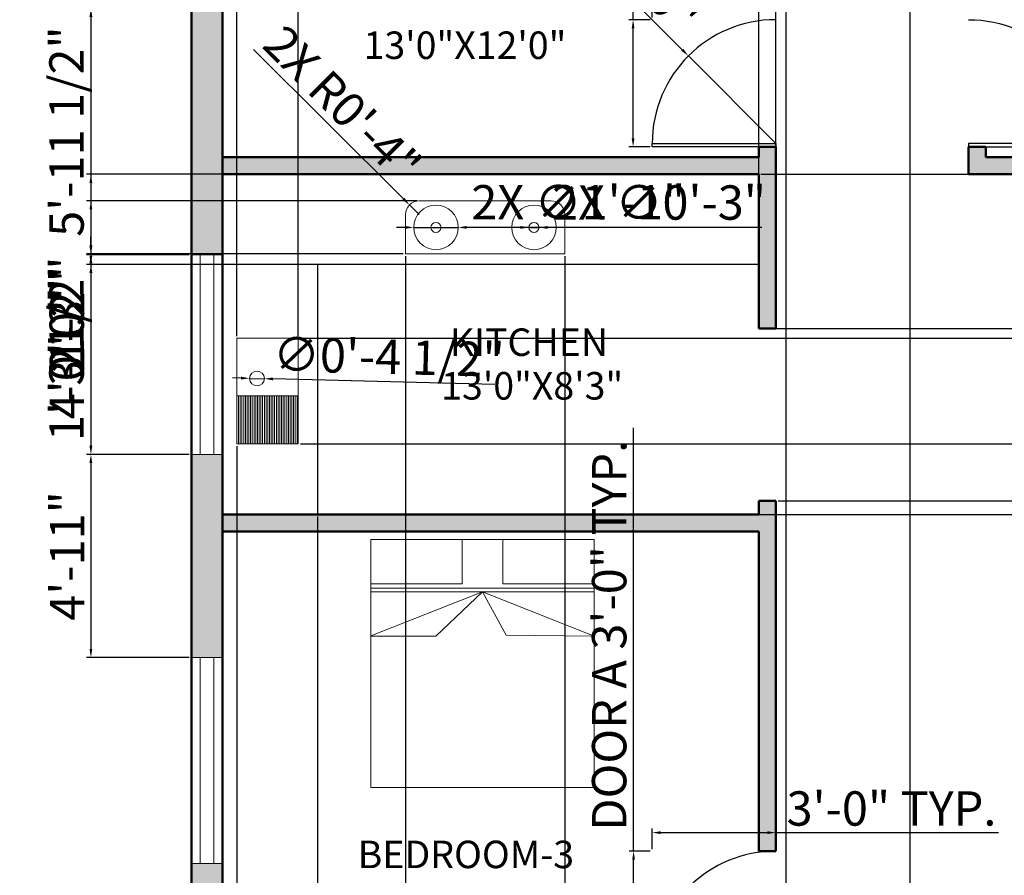
# Model space of a CAD drawing. Units: inches. Extents: x 2719 to 3167, y 1639 to 2327.
# Tile 2 of 4: x 2719 to 3005, y 1881 to 2130. Entities that reach past the tile are written whole.
import ezdxf

# ---------------------------------------------------------------- set-up
doc = ezdxf.new("R2010")
doc.units = ezdxf.units.IN
for name, color, linetype, lineweight in [('A-ANNO-DIMS', 121, 'Continuous', 18), ('A-AREA-IDEN', 121, 'Continuous', 18), ('A-DOOR', 50, 'Continuous', 25), ('A-EQPM', 211, 'Continuous', 18), ('A-FLOR-CASE', 211, 'Continuous', 25), ('A-FLOR-FIXT', 211, 'Continuous', 18), ('A-FLOR-FIXT-PATT', 211, 'Continuous', 13), ('A-FURN', 211, 'Continuous', 18), ('A-GLAZ', 191, 'Continuous', 18), ('A-WALL', 7, 'Continuous', 50)]:
    doc.layers.add(name, color=color, linetype=linetype, lineweight=lineweight)
doc.layers.add('A-WALL-PATT', color=251, linetype='Continuous', lineweight=13, true_color=0x636466)
doc.styles.get("Standard").update_dxf_attribs({"font": 'arial.ttf'})
doc.dimstyles.new('ISO-25', dxfattribs={"dimtxt": 10, "dimasz": 2.5, "dimexe": 1.25, "dimexo": 0.625, "dimtad": 1, "dimdec": 0, "dimlunit": 3, "dimtxsty": 'Standard', "dimcen": 2.5, "dimadec": 0, "dimazin": 0, "dimtfac": 1, "dimtdec": 0, "dimtmove": 0, "dimatfit": 3, "dimfxl": 1, "dimarcsym": 0})

# ---------------------------------------------------------------- blocks, each defined once
blk = doc.blocks.new('BED-DOUBLE')
for p, q in [((0, 57.96), (64.91, 57.96)), ((0, 56.96), (64.91, 56.96)), ((32.46, 56.96), (0, 44.1)), ((32.46, 56.96), (18.94, 44.05)), ((32.46, 56.96), (64.91, 44.04)), ((32.46, 56.96), (39.4, 44.29)), ((18.94, 44.05), (0, 44.05)), ((39.4, 44.29), (64.91, 44.04))]:
    blk.add_line(p, q)
for points in [[(0, 72.15), (64.91, 72.15), (64.91, 0), (0, 0)], [(0, 72.15), (26.55, 72.15), (26.55, 59.27), (0, 59.27)], [(38.37, 72.15), (64.91, 72.15), (64.91, 59.27), (38.37, 59.27)]]:
    blk.add_lwpolyline(points, close=True)
blk = doc.blocks.new('WIN-60IN')
for p, q in [((9, 60), (0, 60)), ((2.5, 60), (2.5, 0)), ((6.5, 60), (6.5, 0)), ((9, 0), (0, 0))]:
    blk.add_line(p, q)
blk = doc.blocks.new('DOOR-36IN-QUARTER-SWING')
for p, q in [((0, 0), (0, 1)), ((0, 1), (36, 1)), ((36, 0), (0, 0)), ((36, 1), (36, 0))]:
    blk.add_line(p, q)
blk.add_arc((36, 1), 36, 90, 180)
blk = doc.blocks.new('DOOR-36IN-SWING')
for p, q in [((0, 0), (0, 1)), ((0, 1), (36, 1)), ((36, 0), (0, 0)), ((36, 1), (36, 0))]:
    blk.add_line(p, q)
blk.add_arc((35.99, 0), 36, 89.9779, 178.4083)
blk = doc.blocks.new('*D11')
at = {"layer": 'A-ANNO-DIMS', "color": 0, "lineweight": -2, "transparency": 16777216}
for p, q in [((2897.39, 1888.44), (2897.39, 2011.64)), ((2902.17, 1888.44), (2896.14, 1888.44)), ((2897.39, 1854.94), (2897.39, 1885.94)), ((2902.17, 1852.44), (2896.14, 1852.44))]:
    blk.add_line(p, q, dxfattribs=at)
at = {"layer": 'A-ANNO-DIMS', "color": 0, "transparency": 16777216}
for points in [[(2896.98, 1885.94), (2897.81, 1885.94), (2897.39, 1888.44)], [(2896.98, 1854.94), (2897.81, 1854.94), (2897.39, 1852.44)]]:
    blk.add_solid(points, dxfattribs=at)
at = {"layer": 'Defpoints', "color": 0, "transparency": 16777216}
for p in [(2897.39, 1888.44), (2902.8, 1888.44), (2902.8, 1852.44)]:
    blk.add_point(p, dxfattribs=at)
at = {"layer": 'A-ANNO-DIMS', "color": 0, "transparency": 16777216, "insert": (2891.59, 1951.29), "char_height": 10, "attachment_point": 5, "rotation": 90}
blk.add_mtext('DOOR A 3\'-0" TYP.', dxfattribs=at)
blk = doc.blocks.new('*D12')
at = {"layer": 'A-ANNO-DIMS', "color": 0, "lineweight": -2, "transparency": 16777216}
for p, q in [((2902.8, 1889.07), (2902.8, 1895.1)), ((2905.3, 1893.85), (2936.3, 1893.85)), ((2938.8, 1889.07), (2938.8, 1895.1)), ((2938.8, 1893.85), (3003.49, 1893.85))]:
    blk.add_line(p, q, dxfattribs=at)
at = {"layer": 'A-ANNO-DIMS', "color": 0, "transparency": 16777216}
for points in [[(2905.3, 1894.26), (2905.3, 1893.43), (2902.8, 1893.85)], [(2936.3, 1894.26), (2936.3, 1893.43), (2938.8, 1893.85)]]:
    blk.add_solid(points, dxfattribs=at)
at = {"layer": 'Defpoints', "color": 0, "transparency": 16777216}
for p in [(2938.8, 1893.85), (2902.8, 1888.44), (2938.8, 1888.44)]:
    blk.add_point(p, dxfattribs=at)
at = {"layer": 'A-ANNO-DIMS', "color": 0, "transparency": 16777216, "insert": (2972.4, 1899.58), "char_height": 10, "attachment_point": 5}
blk.add_mtext('3\'-0" TYP.', dxfattribs=at)
blk = doc.blocks.new('*D13')
at = {"layer": 'A-ANNO-DIMS', "color": 0, "lineweight": -2, "transparency": 16777216}
for p, q in [((2897.25, 2130.44), (2897.25, 2253.63)), ((2902.17, 2130.44), (2896, 2130.44)), ((2897.25, 2095.94), (2897.25, 2127.94)), ((2902.17, 2093.44), (2896, 2093.44))]:
    blk.add_line(p, q, dxfattribs=at)
at = {"layer": 'A-ANNO-DIMS', "color": 0, "transparency": 16777216}
for points in [[(2896.83, 2127.94), (2897.66, 2127.94), (2897.25, 2130.44)], [(2896.83, 2095.94), (2897.66, 2095.94), (2897.25, 2093.44)]]:
    blk.add_solid(points, dxfattribs=at)
at = {"layer": 'Defpoints', "color": 0, "transparency": 16777216}
for p in [(2897.25, 2130.44), (2902.8, 2130.44), (2902.8, 2093.44)]:
    blk.add_point(p, dxfattribs=at)
at = {"layer": 'A-ANNO-DIMS', "color": 0, "transparency": 16777216, "insert": (2891.44, 2193.29), "char_height": 10, "attachment_point": 5, "rotation": 90}
blk.add_mtext('DOOR B 3\'-1" TYP.', dxfattribs=at)
blk = doc.blocks.new('*D14')
at = {"layer": 'A-ANNO-DIMS', "color": 0, "lineweight": -2, "transparency": 16777216}
for p, q in [((2902.8, 2131.06), (2902.8, 2137.24)), ((2938.8, 2131.06), (2938.8, 2137.24)), ((2905.3, 2135.99), (2936.3, 2135.99)), ((2938.8, 2135.99), (3003.49, 2135.99))]:
    blk.add_line(p, q, dxfattribs=at)
at = {"layer": 'A-ANNO-DIMS', "color": 0, "transparency": 16777216}
for points in [[(2905.3, 2136.4), (2905.3, 2135.57), (2902.8, 2135.99)], [(2936.3, 2136.4), (2936.3, 2135.57), (2938.8, 2135.99)]]:
    blk.add_solid(points, dxfattribs=at)
at = {"layer": 'Defpoints', "color": 0, "transparency": 16777216}
for p in [(2938.8, 2135.99), (2902.8, 2130.44), (2938.8, 2130.44)]:
    blk.add_point(p, dxfattribs=at)
at = {"layer": 'A-ANNO-DIMS', "color": 0, "transparency": 16777216, "insert": (2972.4, 2141.72), "char_height": 10, "attachment_point": 5}
blk.add_mtext('3\'-0" TYP.', dxfattribs=at)
blk = doc.blocks.new('*D20')
at = {"layer": 'A-ANNO-DIMS', "color": 0, "lineweight": -2, "transparency": 16777216}
for p, q in [((2768.17, 2133.72), (2738.3, 2133.72)), ((2739.55, 2131.22), (2739.55, 2064.55)), ((2768.17, 2062.05), (2738.3, 2062.05))]:
    blk.add_line(p, q, dxfattribs=at)
at = {"layer": 'A-ANNO-DIMS', "color": 0, "transparency": 16777216}
for points in [[(2739.13, 2131.22), (2739.96, 2131.22), (2739.55, 2133.72)], [(2739.13, 2064.55), (2739.96, 2064.55), (2739.55, 2062.05)]]:
    blk.add_solid(points, dxfattribs=at)
at = {"layer": 'Defpoints', "color": 0, "transparency": 16777216}
for p in [(2768.8, 2133.72), (2739.55, 2062.05), (2768.8, 2062.05)]:
    blk.add_point(p, dxfattribs=at)
at = {"layer": 'A-ANNO-DIMS', "color": 0, "transparency": 16777216, "insert": (2733.75, 2097.88), "char_height": 10, "attachment_point": 5, "rotation": 90}
blk.add_mtext('5\'-11 1/2"', dxfattribs=at)
blk = doc.blocks.new('*D21')
at = {"layer": 'A-ANNO-DIMS', "color": 0, "lineweight": -2, "transparency": 16777216}
for p, q in [((2768.17, 2062.05), (2738.3, 2062.05)), ((2739.55, 2059.55), (2739.55, 2006.42)), ((2768.17, 2003.92), (2738.3, 2003.92))]:
    blk.add_line(p, q, dxfattribs=at)
at = {"layer": 'A-ANNO-DIMS', "color": 0, "transparency": 16777216}
for points in [[(2739.13, 2059.55), (2739.96, 2059.55), (2739.55, 2062.05)], [(2739.13, 2006.42), (2739.96, 2006.42), (2739.55, 2003.92)]]:
    blk.add_solid(points, dxfattribs=at)
at = {"layer": 'Defpoints', "color": 0, "transparency": 16777216}
for p in [(2768.8, 2062.05), (2739.55, 2003.92), (2768.8, 2003.92)]:
    blk.add_point(p, dxfattribs=at)
at = {"layer": 'A-ANNO-DIMS', "color": 0, "transparency": 16777216, "insert": (2733.82, 2032.98), "char_height": 10, "attachment_point": 5, "rotation": 90}
blk.add_mtext('4\'-10"', dxfattribs=at)
blk = doc.blocks.new('*D22')
at = {"layer": 'A-ANNO-DIMS', "color": 0, "lineweight": -2, "transparency": 16777216}
for p, q in [((2768.17, 2003.92), (2738.3, 2003.92)), ((2739.55, 2001.42), (2739.55, 1947.33)), ((2768.17, 1944.83), (2738.3, 1944.83))]:
    blk.add_line(p, q, dxfattribs=at)
at = {"layer": 'A-ANNO-DIMS', "color": 0, "transparency": 16777216}
for points in [[(2739.13, 2001.42), (2739.96, 2001.42), (2739.55, 2003.92)], [(2739.13, 1947.33), (2739.96, 1947.33), (2739.55, 1944.83)]]:
    blk.add_solid(points, dxfattribs=at)
at = {"layer": 'Defpoints', "color": 0, "transparency": 16777216}
for p in [(2768.8, 2003.92), (2739.55, 1944.83), (2768.8, 1944.83)]:
    blk.add_point(p, dxfattribs=at)
at = {"layer": 'A-ANNO-DIMS', "color": 0, "transparency": 16777216, "insert": (2733.9, 1974.37), "char_height": 10, "attachment_point": 5, "rotation": 90}
blk.add_mtext('4\'-11"', dxfattribs=at)
blk = doc.blocks.new('*D28')
at = {"layer": 'A-ANNO-DIMS', "color": 0, "lineweight": -2, "transparency": 16777216}
for p, q in [((2933.8, 2041.15), (2933.8, 2273.94)), ((2938.8, 2041.15), (2938.8, 2273.94)), ((2931.3, 2272.69), (2928.8, 2272.69)), ((2933.8, 2272.69), (2938.8, 2272.69)), ((2941.3, 2272.69), (2971.63, 2272.69))]:
    blk.add_line(p, q, dxfattribs=at)
at = {"layer": 'A-ANNO-DIMS', "color": 0, "transparency": 16777216}
for points in [[(2931.3, 2273.1), (2931.3, 2272.27), (2933.8, 2272.69)], [(2941.3, 2273.1), (2941.3, 2272.27), (2938.8, 2272.69)]]:
    blk.add_solid(points, dxfattribs=at)
at = {"layer": 'Defpoints', "color": 0, "transparency": 16777216}
for p in [(2938.8, 2272.69), (2933.8, 2040.53), (2938.8, 2040.53)]:
    blk.add_point(p, dxfattribs=at)
at = {"layer": 'A-ANNO-DIMS', "color": 0, "transparency": 16777216, "insert": (2957.71, 2278.42), "char_height": 10, "attachment_point": 5}
blk.add_mtext('0\'-5"', dxfattribs=at)
blk = doc.blocks.new('*D29')
at = {"layer": 'A-ANNO-DIMS', "color": 0, "lineweight": -2, "transparency": 16777216}
for p, q in [((2939.42, 2040.53), (3159.3, 2040.53)), ((3158.05, 2038.03), (3158.05, 1992.94)), ((2939.42, 1990.44), (3159.3, 1990.44))]:
    blk.add_line(p, q, dxfattribs=at)
at = {"layer": 'A-ANNO-DIMS', "color": 0, "transparency": 16777216}
for points in [[(3157.63, 2038.03), (3158.46, 2038.03), (3158.05, 2040.53)], [(3157.63, 1992.94), (3158.46, 1992.94), (3158.05, 1990.44)]]:
    blk.add_solid(points, dxfattribs=at)
at = {"layer": 'Defpoints', "color": 0, "transparency": 16777216}
for p in [(2938.8, 2040.53), (2938.8, 1990.44), (3158.05, 1990.44)]:
    blk.add_point(p, dxfattribs=at)
at = {"layer": 'A-ANNO-DIMS', "color": 0, "transparency": 16777216, "insert": (3152.4, 2015.48), "char_height": 10, "attachment_point": 5, "rotation": 90}
blk.add_mtext('4\'-2"', dxfattribs=at)
blk = doc.blocks.new('*D30')
at = {"layer": 'A-ANNO-DIMS', "color": 0, "lineweight": -2, "transparency": 16777216}
for p, q in [((2934.42, 2085.44), (3159.3, 2085.44)), ((3158.05, 2082.94), (3158.05, 2043.03)), ((2934.42, 2040.53), (3159.3, 2040.53))]:
    blk.add_line(p, q, dxfattribs=at)
at = {"layer": 'A-ANNO-DIMS', "color": 0, "transparency": 16777216}
for points in [[(3157.63, 2082.94), (3158.46, 2082.94), (3158.05, 2085.44)], [(3157.63, 2043.03), (3158.46, 2043.03), (3158.05, 2040.53)]]:
    blk.add_solid(points, dxfattribs=at)
at = {"layer": 'Defpoints', "color": 0, "transparency": 16777216}
for p in [(2933.8, 2085.44), (2933.8, 2040.53), (3158.05, 2040.53)]:
    blk.add_point(p, dxfattribs=at)
at = {"layer": 'A-ANNO-DIMS', "color": 0, "transparency": 16777216, "insert": (3152.31, 2062.98), "char_height": 10, "attachment_point": 5, "rotation": 90}
blk.add_mtext('3\'-9"', dxfattribs=at)
blk = doc.blocks.new('*D31')
at = {"layer": 'A-ANNO-DIMS', "color": 0, "lineweight": -2, "transparency": 16777216}
for p, q in [((2777.8, 1985.81), (2777.8, 1672.94)), ((2805.5, 1985.81), (2805.5, 1672.94)), ((2780.3, 1674.19), (2803, 1674.19)), ((2805.5, 1674.19), (2859.31, 1674.19))]:
    blk.add_line(p, q, dxfattribs=at)
at = {"layer": 'A-ANNO-DIMS', "color": 0, "transparency": 16777216}
for points in [[(2780.3, 1674.6), (2780.3, 1673.77), (2777.8, 1674.19)], [(2803, 1674.6), (2803, 1673.77), (2805.5, 1674.19)]]:
    blk.add_solid(points, dxfattribs=at)
at = {"layer": 'Defpoints', "color": 0, "transparency": 16777216}
for p in [(2777.8, 1986.44), (2805.5, 1986.44), (2805.5, 1674.19)]:
    blk.add_point(p, dxfattribs=at)
at = {"layer": 'A-ANNO-DIMS', "color": 0, "transparency": 16777216, "insert": (2833.65, 1679.99), "char_height": 10, "attachment_point": 5}
blk.add_mtext('2\'-3 1/2"', dxfattribs=at)
blk = doc.blocks.new('*D32')
at = {"layer": 'A-ANNO-DIMS', "color": 0, "lineweight": -2, "transparency": 16777216}
for p, q in [((2933.17, 2085.44), (2738.3, 2085.44)), ((2739.55, 2082.94), (2739.55, 2061.71)), ((2933.17, 2059.21), (2738.3, 2059.21)), ((2739.55, 2059.21), (2739.55, 2028.71))]:
    blk.add_line(p, q, dxfattribs=at)
at = {"layer": 'A-ANNO-DIMS', "color": 0, "transparency": 16777216}
for points in [[(2739.13, 2082.94), (2739.96, 2082.94), (2739.55, 2085.44)], [(2739.13, 2061.71), (2739.96, 2061.71), (2739.55, 2059.21)]]:
    blk.add_solid(points, dxfattribs=at)
at = {"layer": 'Defpoints', "color": 0, "transparency": 16777216}
for p in [(2933.8, 2085.44), (2739.55, 2059.21), (2933.8, 2059.21)]:
    blk.add_point(p, dxfattribs=at)
at = {"layer": 'A-ANNO-DIMS', "color": 0, "transparency": 16777216, "insert": (2733.9, 2042.71), "char_height": 10, "attachment_point": 5, "rotation": 90}
blk.add_mtext('2\'-2"', dxfattribs=at)
blk = doc.blocks.new('*D33')
at = {"layer": 'A-ANNO-DIMS', "color": 0, "lineweight": -2, "transparency": 16777216}
for p, q in [((2782.04, 2038.37), (2782.04, 2273.94)), ((2799.85, 2038.37), (2799.85, 2273.94)), ((2784.54, 2272.69), (2797.35, 2272.69)), ((2799.85, 2272.69), (2829.24, 2272.69))]:
    blk.add_line(p, q, dxfattribs=at)
at = {"layer": 'A-ANNO-DIMS', "color": 0, "transparency": 16777216}
for points in [[(2784.54, 2273.1), (2784.54, 2272.27), (2782.04, 2272.69)], [(2797.35, 2273.1), (2797.35, 2272.27), (2799.85, 2272.69)]]:
    blk.add_solid(points, dxfattribs=at)
at = {"layer": 'Defpoints', "color": 0, "transparency": 16777216}
for p in [(2799.85, 2272.69), (2782.04, 2037.74), (2799.85, 2037.74)]:
    blk.add_point(p, dxfattribs=at)
at = {"layer": 'A-ANNO-DIMS', "color": 0, "transparency": 16777216, "insert": (2815.79, 2278.42), "char_height": 10, "attachment_point": 5}
blk.add_mtext('1\'-6"', dxfattribs=at)
blk = doc.blocks.new('*D34')
at = {"layer": 'A-ANNO-DIMS', "color": 0, "lineweight": -2, "transparency": 16777216}
for p, q in [((2800.47, 2037.74), (3159.3, 2037.74)), ((3158.05, 2035.24), (3158.05, 2009.46)), ((2800.47, 2006.96), (3159.3, 2006.96))]:
    blk.add_line(p, q, dxfattribs=at)
at = {"layer": 'A-ANNO-DIMS', "color": 0, "transparency": 16777216}
for points in [[(3157.63, 2035.24), (3158.46, 2035.24), (3158.05, 2037.74)], [(3157.63, 2009.46), (3158.46, 2009.46), (3158.05, 2006.96)]]:
    blk.add_solid(points, dxfattribs=at)
at = {"layer": 'Defpoints', "color": 0, "transparency": 16777216}
for p in [(2799.85, 2037.74), (2799.85, 2006.96), (3158.05, 2006.96)]:
    blk.add_point(p, dxfattribs=at)
at = {"layer": 'A-ANNO-DIMS', "color": 0, "transparency": 16777216, "insert": (3152.4, 2022.35), "char_height": 10, "attachment_point": 5, "rotation": 90}
blk.add_mtext('2\'-7"', dxfattribs=at)
blk = doc.blocks.new('*D35')
at = {"layer": 'A-ANNO-DIMS', "color": 0, "lineweight": -2, "transparency": 16777216}
for p, q in [((2800.47, 2006.96), (3159.3, 2006.96)), ((3158.05, 2004.46), (3158.05, 1988.94)), ((2806.13, 1986.44), (3159.3, 1986.44)), ((3158.05, 1986.44), (3158.05, 1933.74))]:
    blk.add_line(p, q, dxfattribs=at)
at = {"layer": 'A-ANNO-DIMS', "color": 0, "transparency": 16777216}
for points in [[(3157.63, 2004.46), (3158.46, 2004.46), (3158.05, 2006.96)], [(3157.63, 1988.94), (3158.46, 1988.94), (3158.05, 1986.44)]]:
    blk.add_solid(points, dxfattribs=at)
at = {"layer": 'Defpoints', "color": 0, "transparency": 16777216}
for p in [(2799.85, 2006.96), (2805.5, 1986.44), (3158.05, 1986.44)]:
    blk.add_point(p, dxfattribs=at)
at = {"layer": 'A-ANNO-DIMS', "color": 0, "transparency": 16777216, "insert": (3152.25, 1958.84), "char_height": 10, "attachment_point": 5, "rotation": 90}
blk.add_mtext('1\'-8 1/2"', dxfattribs=at)
blk = doc.blocks.new('*D36')
at = {"layer": 'A-ANNO-DIMS', "color": 0, "lineweight": -2, "transparency": 16777216}
for p, q in [((2782.04, 2006.33), (2782.04, 1672.94)), ((2777.8, 1985.81), (2777.8, 1672.94)), ((2775.3, 1674.19), (2744.96, 1674.19)), ((2782.04, 1674.19), (2777.8, 1674.19)), ((2784.54, 1674.19), (2787.04, 1674.19))]:
    blk.add_line(p, q, dxfattribs=at)
at = {"layer": 'A-ANNO-DIMS', "color": 0, "transparency": 16777216}
for points in [[(2775.3, 1674.6), (2775.3, 1673.77), (2777.8, 1674.19)], [(2784.54, 1674.6), (2784.54, 1673.77), (2782.04, 1674.19)]]:
    blk.add_solid(points, dxfattribs=at)
at = {"layer": 'Defpoints', "color": 0, "transparency": 16777216}
for p in [(2782.04, 2006.96), (2777.8, 1986.44), (2777.8, 1674.19)]:
    blk.add_point(p, dxfattribs=at)
at = {"layer": 'A-ANNO-DIMS', "color": 0, "transparency": 16777216, "insert": (2758.88, 1679.92), "char_height": 10, "attachment_point": 5}
blk.add_mtext('0\'-4"', dxfattribs=at)
blk = doc.blocks.new('*D37')
at = {"layer": 'A-ANNO-DIMS', "color": 0, "lineweight": -2, "transparency": 16777216}
for p, q in [((2831.04, 2061.64), (2831.04, 1672.94)), ((2877.4, 2061.64), (2877.4, 1672.94)), ((2833.54, 1674.19), (2874.9, 1674.19)), ((2877.4, 1674.19), (2938.79, 1674.19))]:
    blk.add_line(p, q, dxfattribs=at)
at = {"layer": 'A-ANNO-DIMS', "color": 0, "transparency": 16777216}
for points in [[(2833.54, 1674.6), (2833.54, 1673.77), (2831.04, 1674.19)], [(2874.9, 1674.6), (2874.9, 1673.77), (2877.4, 1674.19)]]:
    blk.add_solid(points, dxfattribs=at)
at = {"layer": 'Defpoints', "color": 0, "transparency": 16777216}
for p in [(2831.04, 2062.26), (2877.4, 2062.26), (2877.4, 1674.19)]:
    blk.add_point(p, dxfattribs=at)
at = {"layer": 'A-ANNO-DIMS', "color": 0, "transparency": 16777216, "insert": (2909.34, 1679.99), "char_height": 10, "attachment_point": 5}
blk.add_mtext('3\'-10 1/2"', dxfattribs=at)
blk = doc.blocks.new('*D38')
at = {"layer": 'A-ANNO-DIMS', "color": 0, "lineweight": -2, "transparency": 16777216}
for p, q in [((2834.42, 2077.7), (2738.3, 2077.7)), ((2739.55, 2075.2), (2739.55, 2064.76)), ((2830.42, 2062.26), (2738.3, 2062.26)), ((2739.55, 2062.26), (2739.55, 2009.57))]:
    blk.add_line(p, q, dxfattribs=at)
at = {"layer": 'A-ANNO-DIMS', "color": 0, "transparency": 16777216}
for points in [[(2739.13, 2075.2), (2739.96, 2075.2), (2739.55, 2077.7)], [(2739.13, 2064.76), (2739.96, 2064.76), (2739.55, 2062.26)]]:
    blk.add_solid(points, dxfattribs=at)
at = {"layer": 'Defpoints', "color": 0, "transparency": 16777216}
for p in [(2835.04, 2077.7), (2739.55, 2062.26), (2831.04, 2062.26)]:
    blk.add_point(p, dxfattribs=at)
at = {"layer": 'A-ANNO-DIMS', "color": 0, "transparency": 16777216, "insert": (2733.75, 2034.67), "char_height": 10, "attachment_point": 5, "rotation": 90}
blk.add_mtext('1\'-3 1/2"', dxfattribs=at)
blk = doc.blocks.new('*D39')
at = {"layer": 'A-ANNO-DIMS', "color": 0, "lineweight": -2, "transparency": 16777216}
for p, q in [((2777.8, 2084.81), (2777.8, 1672.94)), ((2831.04, 2061.64), (2831.04, 1672.94)), ((2780.3, 1674.19), (2828.54, 1674.19))]:
    blk.add_line(p, q, dxfattribs=at)
at = {"layer": 'A-ANNO-DIMS', "color": 0, "transparency": 16777216}
for points in [[(2780.3, 1674.6), (2780.3, 1673.77), (2777.8, 1674.19)], [(2828.54, 1674.6), (2828.54, 1673.77), (2831.04, 1674.19)]]:
    blk.add_solid(points, dxfattribs=at)
at = {"layer": 'Defpoints', "color": 0, "transparency": 16777216}
for p in [(2777.8, 2085.44), (2831.04, 2062.26), (2831.04, 1674.19)]:
    blk.add_point(p, dxfattribs=at)
at = {"layer": 'A-ANNO-DIMS', "color": 0, "transparency": 16777216, "insert": (2804.42, 1679.9), "char_height": 10, "attachment_point": 5}
blk.add_mtext('4\'-5"', dxfattribs=at)
blk = doc.blocks.new('*D40')
at = {"layer": 'A-ANNO-DIMS', "color": 0, "lineweight": -2, "transparency": 16777216}
for p, q in [((2739.55, 2064.76), (2739.55, 2067.26)), ((2830.42, 2062.26), (2738.3, 2062.26)), ((2739.55, 2062.26), (2739.55, 2059.21)), ((2804.88, 2059.21), (2738.3, 2059.21)), ((2739.55, 2056.71), (2739.55, 2026.38))]:
    blk.add_line(p, q, dxfattribs=at)
at = {"layer": 'A-ANNO-DIMS', "color": 0, "transparency": 16777216}
for points in [[(2739.13, 2064.76), (2739.96, 2064.76), (2739.55, 2062.26)], [(2739.13, 2056.71), (2739.96, 2056.71), (2739.55, 2059.21)]]:
    blk.add_solid(points, dxfattribs=at)
at = {"layer": 'Defpoints', "color": 0, "transparency": 16777216}
for p in [(2831.04, 2062.26), (2739.55, 2059.21), (2805.5, 2059.21)]:
    blk.add_point(p, dxfattribs=at)
at = {"layer": 'A-ANNO-DIMS', "color": 0, "transparency": 16777216, "insert": (2733.81, 2040.29), "char_height": 10, "attachment_point": 5, "rotation": 90}
blk.add_mtext('0\'-3"', dxfattribs=at)
blk = doc.blocks.new('*D48')
at = {"layer": 'A-ANNO-DIMS', "color": 0, "lineweight": -2, "transparency": 16777216}
for p, q in [((2941.8, 1796.06), (2941.8, 2273.94)), ((2977.8, 1796.06), (2977.8, 2273.94)), ((2944.3, 2272.69), (2975.3, 2272.69))]:
    blk.add_line(p, q, dxfattribs=at)
at = {"layer": 'A-ANNO-DIMS', "color": 0, "transparency": 16777216}
for points in [[(2944.3, 2273.1), (2944.3, 2272.27), (2941.8, 2272.69)], [(2975.3, 2273.1), (2975.3, 2272.27), (2977.8, 2272.69)]]:
    blk.add_solid(points, dxfattribs=at)
at = {"layer": 'Defpoints', "color": 0, "transparency": 16777216}
for p in [(2977.8, 2272.69), (2941.8, 1795.44), (2977.8, 1795.44)]:
    blk.add_point(p, dxfattribs=at)
at = {"layer": 'A-ANNO-DIMS', "color": 0, "transparency": 16777216, "insert": (2959.8, 2278.42), "char_height": 10, "attachment_point": 5}
blk.add_mtext('3\'-0"', dxfattribs=at)
blk = doc.blocks.new('*D54')
at = {"layer": 'A-ANNO-DIMS', "color": 0, "lineweight": -2, "transparency": 16777216}
for p, q in [((2868.04, 2165.19), (2911.57, 2121.66)), ((2938.8, 2094.44), (2913.34, 2119.89))]:
    blk.add_line(p, q, dxfattribs=at)
at = {"layer": 'A-ANNO-DIMS', "color": 0, "transparency": 16777216}
blk.add_solid([(2911.87, 2121.96), (2911.28, 2121.37), (2913.34, 2119.89)], dxfattribs=at)
at = {"layer": 'Defpoints', "color": 0, "transparency": 16777216}
for p in [(2913.34, 2119.89), (2938.8, 2094.44)]:
    blk.add_point(p, dxfattribs=at)
at = {"layer": 'A-ANNO-DIMS', "color": 0, "transparency": 16777216, "insert": (2892.98, 2148.36), "char_height": 10, "attachment_point": 5, "rotation": 315.0006}
blk.add_mtext('2X R3\'-0"', dxfattribs=at)
blk = doc.blocks.new('*D56')
at = {"layer": 'A-ANNO-DIMS', "color": 0, "lineweight": -2, "transparency": 16777216}
for p, q in [((2830.93, 2069.98), (2828.43, 2069.98)), ((2833.43, 2069.98), (2846.38, 2069.98)), ((2911.22, 2069.99), (2848.88, 2069.98))]:
    blk.add_line(p, q, dxfattribs=at)
at = {"layer": 'A-ANNO-DIMS', "color": 0, "transparency": 16777216}
for points in [[(2830.93, 2070.4), (2830.93, 2069.56), (2833.43, 2069.98)], [(2848.88, 2070.4), (2848.88, 2069.57), (2846.38, 2069.98)]]:
    blk.add_solid(points, dxfattribs=at)
at = {"layer": 'Defpoints', "color": 0, "transparency": 16777216}
for p in [(2833.43, 2069.98), (2846.38, 2069.98)]:
    blk.add_point(p, dxfattribs=at)
at = {"layer": 'A-ANNO-DIMS', "color": 0, "transparency": 16777216, "insert": (2881.3, 2076), "char_height": 10, "attachment_point": 5, "rotation": 0.0043}
blk.add_mtext('2X ∅1\'-1"', dxfattribs=at)
blk = doc.blocks.new('*D58')
at = {"layer": 'A-ANNO-DIMS', "color": 0, "lineweight": -2, "transparency": 16777216}
for p, q in [((2864.45, 2069.99), (2861.95, 2069.99)), ((2866.95, 2069.98), (2869.89, 2069.98)), ((2934.73, 2069.91), (2872.39, 2069.98))]:
    blk.add_line(p, q, dxfattribs=at)
at = {"layer": 'A-ANNO-DIMS', "color": 0, "transparency": 16777216}
for points in [[(2864.45, 2070.4), (2864.45, 2069.57), (2866.95, 2069.98)], [(2872.39, 2070.39), (2872.39, 2069.56), (2869.89, 2069.98)]]:
    blk.add_solid(points, dxfattribs=at)
at = {"layer": 'Defpoints', "color": 0, "transparency": 16777216}
for p in [(2866.95, 2069.98), (2869.89, 2069.98)]:
    blk.add_point(p, dxfattribs=at)
at = {"layer": 'A-ANNO-DIMS', "color": 0, "transparency": 16777216, "insert": (2904.81, 2075.95), "char_height": 10, "attachment_point": 5, "rotation": 359.9408}
blk.add_mtext('2X ∅0\'-3"', dxfattribs=at)
blk = doc.blocks.new('*D59')
at = {"layer": 'A-ANNO-DIMS', "color": 0, "lineweight": -2, "transparency": 16777216}
for p, q in [((2783.22, 2026.13), (2780.72, 2026.19)), ((2785.72, 2026.06), (2790.01, 2025.95)), ((2857, 2024.23), (2792.51, 2025.89))]:
    blk.add_line(p, q, dxfattribs=at)
at = {"layer": 'A-ANNO-DIMS', "color": 0, "transparency": 16777216}
for points in [[(2783.23, 2026.55), (2783.21, 2025.71), (2785.72, 2026.06)], [(2792.52, 2026.31), (2792.5, 2025.47), (2790.01, 2025.95)]]:
    blk.add_solid(points, dxfattribs=at)
at = {"layer": 'Defpoints', "color": 0, "transparency": 16777216}
for p in [(2785.72, 2026.06), (2790.01, 2025.95)]:
    blk.add_point(p, dxfattribs=at)
at = {"layer": 'A-ANNO-DIMS', "color": 0, "transparency": 16777216, "insert": (2826.16, 2031.03), "char_height": 10, "attachment_point": 5, "rotation": 358.5229}
blk.add_mtext('∅0\'-4 1/2"', dxfattribs=at)
blk = doc.blocks.new('*D60')
at = {"layer": 'A-ANNO-DIMS', "color": 0, "lineweight": -2, "transparency": 16777216}
for p, q in [((2786.88, 2121.79), (2830.44, 2078.29)), ((2835.04, 2073.7), (2832.21, 2076.53))]:
    blk.add_line(p, q, dxfattribs=at)
at = {"layer": 'A-ANNO-DIMS', "color": 0, "transparency": 16777216}
blk.add_solid([(2830.74, 2078.59), (2830.15, 2078), (2832.21, 2076.53)], dxfattribs=at)
at = {"layer": 'Defpoints', "color": 0, "transparency": 16777216}
for p in [(2832.21, 2076.53), (2835.04, 2073.7)]:
    blk.add_point(p, dxfattribs=at)
at = {"layer": 'A-ANNO-DIMS', "color": 0, "transparency": 16777216, "insert": (2811.83, 2104.98), "char_height": 10, "attachment_point": 5, "rotation": 315.044}
blk.add_mtext('2X R0\'-4"', dxfattribs=at)

msp = doc.modelspace()

# ---------------------------------------------------------------- hatches: boundary and pattern name
at = {"layer": 'A-FLOR-FIXT-PATT'}
h = msp.add_hatch(dxfattribs=at)
h.set_pattern_fill('ANSI31', color=256, scale=0.15748, angle=45, style=0)
h.paths.add_polyline_path([(2782.04, 2006.96), (2799.85, 2006.96), (2799.85, 2021), (2782.04, 2021)])
at = {"layer": 'A-WALL-PATT'}
h = msp.add_hatch(color=256, dxfattribs=at)
h.dxf.hatch_style = 1
h.paths.add_polyline_path([(2777.8, 2133.72), (2768.8, 2133.72), (2768.8, 2062.05), (2777.8, 2062.05)])
h = msp.add_hatch(color=256, dxfattribs=at)
h.dxf.hatch_style = 1
h.paths.add_polyline_path([(2938.8, 2090.44), (2938.8, 2093.44), (2933.8, 2093.44), (2933.8, 2090.44), (2777.8, 2090.44), (2777.8, 2085.44), (2933.8, 2085.44), (2933.8, 2040.53), (2938.8, 2040.53)])
h = msp.add_hatch(color=256, dxfattribs=at)
h.dxf.hatch_style = 1
h.paths.add_polyline_path([(3119.8, 2090.44), (2999.8, 2090.44), (2999.8, 2093.44), (2994.8, 2093.44), (2994.8, 2090.44), (2994.8, 2085.44), (3119.8, 2085.44)])
h = msp.add_hatch(color=256, dxfattribs=at)
h.dxf.hatch_style = 1
h.paths.add_polyline_path([(2777.8, 2003.92), (2768.8, 2003.92), (2768.8, 1944.83), (2777.8, 1944.83)])
h = msp.add_hatch(color=256, dxfattribs=at)
h.dxf.hatch_style = 1
h.paths.add_polyline_path([(2938.8, 1990.44), (2933.8, 1990.44), (2933.8, 1986.44), (2777.8, 1986.44), (2777.8, 1981.44), (2933.8, 1981.44), (2933.8, 1888.44), (2938.8, 1888.44)])
h = msp.add_hatch(color=256, dxfattribs=at)
h.dxf.hatch_style = 1
h.paths.add_polyline_path([(2777.8, 1884.83), (2768.8, 1884.83), (2768.8, 1703.44), (2823.4, 1703.44), (2823.4, 1712.44), (2777.8, 1712.44)])

# ---------------------------------------------------------------- linework, layer by layer
at = {"layer": 'A-EQPM'}
msp.add_lwpolyline([(2835.04, 2077.7), (2873.4, 2077.7, -0.414214), (2877.4, 2073.7), (2877.4, 2062.26), (2831.04, 2062.26), (2831.04, 2073.7, -0.414214)], format="xyb", close=True, dxfattribs=at)
for centre, radius in [((2839.91, 2069.98), 6.48), ((2868.42, 2069.98), 6.48), ((2839.91, 2069.98), 1.47), ((2868.42, 2069.98), 1.47)]:
    msp.add_circle(centre, radius, dxfattribs=at)
at = {"layer": 'A-FLOR-CASE'}
for p, q in [((2933.8, 2059.21), (2805.5, 2059.21)), ((2805.5, 2059.21), (2805.5, 1986.44))]:
    msp.add_line(p, q, dxfattribs=at)
at = {"layer": 'A-FLOR-FIXT'}
msp.add_line((2782.04, 2021), (2799.85, 2021), dxfattribs=at)
msp.add_lwpolyline([(2782.04, 2037.74), (2799.85, 2037.74), (2799.85, 2006.96), (2782.04, 2006.96)], close=True, dxfattribs=at)
msp.add_circle((2787.86, 2026.01), 2.15, dxfattribs=at)
at = {"layer": 'A-GLAZ'}
for p, q in [((2768.8, 2062.05), (2777.8, 2062.05)), ((2771.3, 2062.05), (2771.3, 2003.92)), ((2775.3, 2062.05), (2775.3, 2003.92)), ((2777.8, 2003.92), (2768.8, 2003.92))]:
    msp.add_line(p, q, dxfattribs=at)
at = {"layer": 'A-WALL'}
for p, q in [((2777.8, 1712.44), (2777.8, 2234.44)), ((2938.8, 2093.44), (2933.8, 2093.44)), ((2933.8, 2093.44), (2933.8, 2090.44)), ((2938.8, 2090.44), (2938.8, 2093.44)), ((2994.8, 2090.44), (2994.8, 2093.44)), ((2994.8, 2093.44), (2999.8, 2093.44)), ((2999.8, 2093.44), (2999.8, 2090.44)), ((2777.8, 2090.44), (2933.8, 2090.44)), ((2938.8, 2040.53), (2938.8, 2090.44)), ((2994.8, 2085.44), (2994.8, 2090.44)), ((2999.8, 2090.44), (3119.8, 2090.44)), ((2777.8, 2085.44), (2933.8, 2085.44)), ((2933.8, 2040.53), (2933.8, 2085.44)), ((2994.8, 2085.44), (3119.8, 2085.44)), ((2933.8, 2040.53), (2938.8, 2040.53)), ((2933.8, 1990.44), (2938.8, 1990.44)), ((2933.8, 1986.44), (2933.8, 1990.44)), ((2938.8, 1888.44), (2938.8, 1990.44)), ((2777.8, 1986.44), (2933.8, 1986.44)), ((2777.8, 1981.44), (2933.8, 1981.44)), ((2933.8, 1888.44), (2933.8, 1981.44)), ((2933.8, 1888.44), (2938.8, 1888.44))]:
    msp.add_line(p, q, dxfattribs=at)
msp.add_lwpolyline([(2941.8, 1703.44), (2768.8, 1703.44), (2768.8, 2243.44), (3128.8, 2243.44), (3128.8, 1703.44), (2989.8, 1703.44)], dxfattribs=at)

# ---------------------------------------------------------------- block references
at = {"layer": 'A-DOOR'}
for name, p in [('DOOR-36IN-QUARTER-SWING', (2902.8, 2093.44)), ('DOOR-36IN-SWING', (2902.8, 1852.44))]:
    msp.add_blockref(name, p, dxfattribs=at)
at = {"layer": 'A-DOOR', "extrusion": (0, 0, -1), "zscale": -1}
msp.add_blockref('DOOR-36IN-QUARTER-SWING', (-3030.8, 2093.44), dxfattribs=at)
at = {"layer": 'A-FURN'}
msp.add_blockref('BED-DOUBLE', (2820.97, 1907), dxfattribs=at)
at = {"layer": 'A-GLAZ', "rotation": 180}
msp.add_blockref('WIN-60IN', (2777.8, 1944.83), dxfattribs=at)

# ---------------------------------------------------------------- texts
at = {"layer": 'A-AREA-IDEN'}
for tag, p in [('13\'0"X12\'0"', (2818.85, 2119)), ('KITCHEN', (2843.93, 2032.58)), ('13\'0"X8\'3"', (2841.43, 2019.88)), ('BEDROOM-3', (2817.14, 1883.51))]:
    msp.add_attdef(tag, p, '', height=8, dxfattribs=at)

# ---------------------------------------------------------------- dimensions: what is measured, and where the dimension line sits
at = {"layer": 'A-ANNO-DIMS'}
for base, p1, p2, picture, middle in [((2799.85, 2272.69), (2782.04, 2037.74), (2799.85, 2037.74), '*D33', (2815.79, 2278.42)), ((2938.8, 2272.69), (2933.8, 2040.53), (2938.8, 2040.53), '*D28', (2957.71, 2278.42)), ((2977.8, 2272.69), (2941.8, 1795.44), (2977.8, 1795.44), '*D48', (2959.8, 2278.42)), ((2831.04, 1674.19), (2777.8, 2085.44), (2831.04, 2062.26), '*D39', (2804.42, 1679.9)), ((2877.4, 1674.19), (2831.04, 2062.26), (2877.4, 2062.26), '*D37', (2909.34, 1679.99)), ((2777.8, 1674.19), (2782.04, 2006.96), (2777.8, 1986.44), '*D36', (2758.88, 1679.92)), ((2805.5, 1674.19), (2777.8, 1986.44), (2805.5, 1986.44), '*D31', (2833.65, 1679.99))]:
    dim = msp.add_linear_dim(base=base, p1=p1, p2=p2, dimstyle='ISO-25', override={"dimdec": 1, "dimlfac": 1, "dimrnd": 0, "dimzin": 1, "dimdsep": 46, "dimlunit": 4, "dimfrac": 2}, dxfattribs=at)
    dim.commit()
    dim.dimension.update_dxf_attribs({"geometry": picture, "text_midpoint": middle})
for base, p1, p2, text, picture, middle in [((2897.25, 2130.44), (2902.8, 2093.44), (2902.8, 2130.44), 'DOOR B <> TYP.', '*D13', (2891.44, 2193.29)), ((2897.39, 1888.44), (2902.8, 1852.44), (2902.8, 1888.44), 'DOOR A <> TYP.', '*D11', (2891.59, 1951.29))]:
    dim = msp.add_linear_dim(base=base, p1=p1, p2=p2, angle=90, text=text, dimstyle='ISO-25', override={"dimdec": 1, "dimlfac": 1, "dimrnd": 0, "dimzin": 1, "dimdsep": 46, "dimlunit": 4, "dimfrac": 2}, dxfattribs=at)
    dim.commit()
    dim.dimension.update_dxf_attribs({"geometry": picture, "text_midpoint": middle})
for center, mpoint, picture, middle in [((2938.8, 2094.44), (2913.34, 2119.89), '*D54', (2892.98, 2148.36)), ((2835.04, 2073.7), (2832.21, 2076.53), '*D60', (2811.83, 2104.98))]:
    dim = msp.add_radius_dim(center=center, mpoint=mpoint, text='2X <>', dimstyle='ISO-25', override={"dimdec": 1, "dimlfac": 1, "dimrnd": 0, "dimzin": 1, "dimdsep": 46, "dimlunit": 4, "dimfrac": 2}, dxfattribs=at)
    dim.commit()
    dim.dimension.update_dxf_attribs({"geometry": picture, "text_midpoint": middle})
for base, p1, p2, picture, middle in [((2938.8, 2135.99), (2902.8, 2130.44), (2938.8, 2130.44), '*D14', (2972.4, 2141.72)), ((2938.8, 1893.85), (2902.8, 1888.44), (2938.8, 1888.44), '*D12', (2972.4, 1899.58))]:
    dim = msp.add_linear_dim(base=base, p1=p1, p2=p2, text='<> TYP.', dimstyle='ISO-25', override={"dimdec": 1, "dimlfac": 1, "dimrnd": 0, "dimzin": 1, "dimdsep": 46, "dimlunit": 4, "dimfrac": 2}, dxfattribs=at)
    dim.commit()
    dim.dimension.update_dxf_attribs({"geometry": picture, "text_midpoint": middle})
for base, p1, p2, picture, middle in [((2739.55, 2062.05), (2768.8, 2133.72), (2768.8, 2062.05), '*D20', (2733.75, 2097.88)), ((2739.55, 2059.21), (2933.8, 2085.44), (2933.8, 2059.21), '*D32', (2733.9, 2042.71)), ((3158.05, 2040.53), (2933.8, 2085.44), (2933.8, 2040.53), '*D30', (3152.31, 2062.98)), ((2739.55, 2062.26), (2835.04, 2077.7), (2831.04, 2062.26), '*D38', (2733.75, 2034.67)), ((2739.5461, 2059.2098), (2831.0443, 2062.263), (2805.502, 2059.2097), '*D40', (2733.8119, 2040.2935)), ((2739.55, 2003.92), (2768.8, 2062.05), (2768.8, 2003.92), '*D21', (2733.82, 2032.98)), ((3158.05, 1990.44), (2938.8, 2040.53), (2938.8, 1990.44), '*D29', (3152.4, 2015.48)), ((3158.05, 2006.96), (2799.85, 2037.74), (2799.85, 2006.96), '*D34', (3152.4, 2022.35)), ((3158.05, 1986.44), (2799.85, 2006.96), (2805.5, 1986.44), '*D35', (3152.25, 1958.84)), ((2739.55, 1944.83), (2768.8, 2003.92), (2768.8, 1944.83), '*D22', (2733.9, 1974.37))]:
    dim = msp.add_linear_dim(base=base, p1=p1, p2=p2, angle=90, dimstyle='ISO-25', override={"dimdec": 1, "dimlfac": 1, "dimrnd": 0, "dimzin": 1, "dimdsep": 46, "dimlunit": 4, "dimfrac": 2}, dxfattribs=at)
    dim.commit()
    dim.dimension.update_dxf_attribs({"geometry": picture, "text_midpoint": middle})
for p1, p2, picture, middle in [((2833.43, 2069.981), (2846.381, 2069.982), '*D56', (2881.3, 2069.9846)), ((2866.95, 2069.98), (2869.89, 2069.98), '*D58', (2904.81, 2069.94))]:
    dim = msp.add_diameter_dim_2p(p1=p1, p2=p2, text='2X <>', dimstyle='ISO-25', override={"dimdec": 1, "dimlfac": 1, "dimrnd": 0, "dimzin": 1, "dimdsep": 46, "dimlunit": 4, "dimfrac": 2}, dxfattribs=at)
    dim.commit()
    dim.dimension.update_dxf_attribs({"geometry": picture, "text_midpoint": middle, "dimtype": 163})
dim = msp.add_diameter_dim_2p(p1=(2785.72, 2026.06), p2=(2790.01, 2025.95), dimstyle='ISO-25', override={"dimdec": 1, "dimlfac": 1, "dimrnd": 0, "dimzin": 1, "dimdsep": 46, "dimlunit": 4, "dimfrac": 2}, dxfattribs=at)
dim.commit()
dim.dimension.update_dxf_attribs({"geometry": '*D59', "text_midpoint": (2826, 2025.03), "dimtype": 163})

doc.saveas('drawing.dxf')
